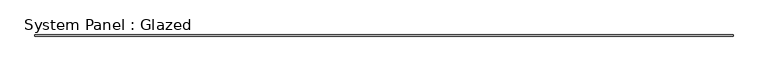
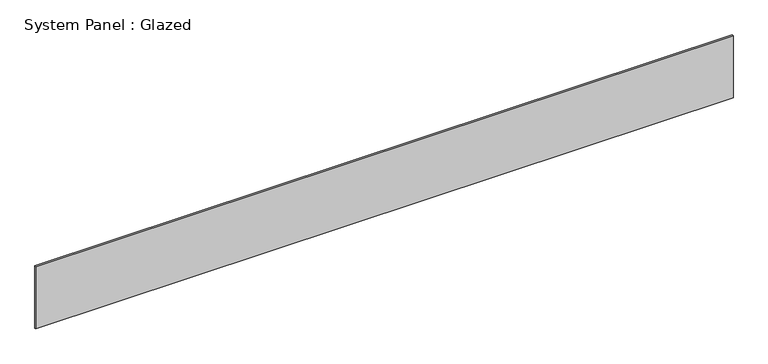
"""IFC4 building model written with IfcOpenShell, lengths in millimetres: plate geometry, System Panel : Glazed."""

from ifc_helpers import new_model, si_unit, origin, origin_with_axes, place, context, project, spatial, polyline, outline, extrude, source, transform, mapped, element, save


def system_panel_glazed_dbf8c7ac(model_context):
    return source(origin(), model_context, "Body", "SweptSolid", [
        extrude(outline(polyline([(8077.2, 19.05), (-8077.2, 19.05), (-8077.2, 44.45), (8077.2, 44.45), (8077.2, 19.05)])), origin_with_axes(), (0.0, 0.0, 1.0), 1524.0),
    ])


if __name__ == "__main__":
    model = new_model("IFC4")
    model_context = context("Model", 3, world=origin())
    ifc_project = project(units=[si_unit("LENGTHUNIT", "METRE", prefix="MILLI")], contexts=[model_context])
    site = spatial("IfcSite", under=ifc_project)
    building = spatial("IfcBuilding", under=site)
    placement = place(None, origin())
    system_panel_glazed_shape = system_panel_glazed_dbf8c7ac(model_context)
    element("IfcPlate", 1, ObjectType="System Panel : Glazed", at=placement, inside=building, context=model_context, shape_type="MappedRepresentation", body=[
        mapped(system_panel_glazed_shape, transform((0.0, 0.0, 0.0), x_axis=(1.0, 0.0, 0.0), y_axis=(0.0, 1.0, 0.0), z_axis=(0.0, 0.0, 1.0))),
    ])
    save(model, "model.ifc")

# Revit data of these elements
# Type "System Panel : Glazed"
#   Construction Type Id = "GSP4R"
#   Analytic Construction = "1/8 in Pilkington single glazing"
#   Visual Light Transmittance = 0.9
#   Solar Heat Gain Coefficient = 0.86
#   Heat Transfer Coefficient (U) = 1.18115 BTU/(h·ft²·°F)
# Element 1 (IfcPlate, "System Panel : Glazed")
#   Materials on its faces: "Glass"
# Materials
#   "Glass": class "Glass", colour RGB 0 128 192, transparency 0.75, Description = "Soda Lime Glass", Cost = 0
